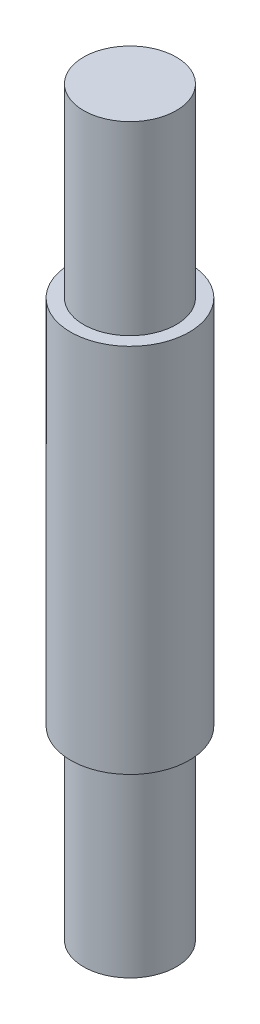
SolidWorks part; units mm, degrees
material "Plain Carbon Steel"
ref_plane "Front Plane" through (0, 0, 0) normal (0, 0, 1) x (1, 0, 0)
ref_plane "Top Plane" through (0, 0, 0) normal (0, 1, 0) x (1, 0, 0)
ref_plane "Right Plane" through (0, 0, 0) normal (1, 0, 0) x (0, 0, -1)
sketch "Pin Profile Sketch" plane through (0, 0, 0) normal (0, 0, 1) x (1, 0, 0)
  line L0 (0, 0) -> (12.5, 0)
  line L1 (12.5, 0) -> (12.5, 50)
  line L2 (12.5, 50) -> (16, 50)
  line L3 (16, 50) -> (16, 150)
  line L4 (16, 150) -> (12.5, 150)
  line L5 (12.5, 150) -> (12.5, 200)
  line L6 (12.5, 200) -> (0, 200)
  line L7 (0, 200) -> (0, 0)
  dimension "D1" = 12.5
  dimension "D2" = 100
  dimension "D3" = 50
  dimension "D4" = 50
  dimension "D5" = 16
revolve "Pin Body Revolve" add sketch "Pin Profile Sketch" angle 360 about L7
